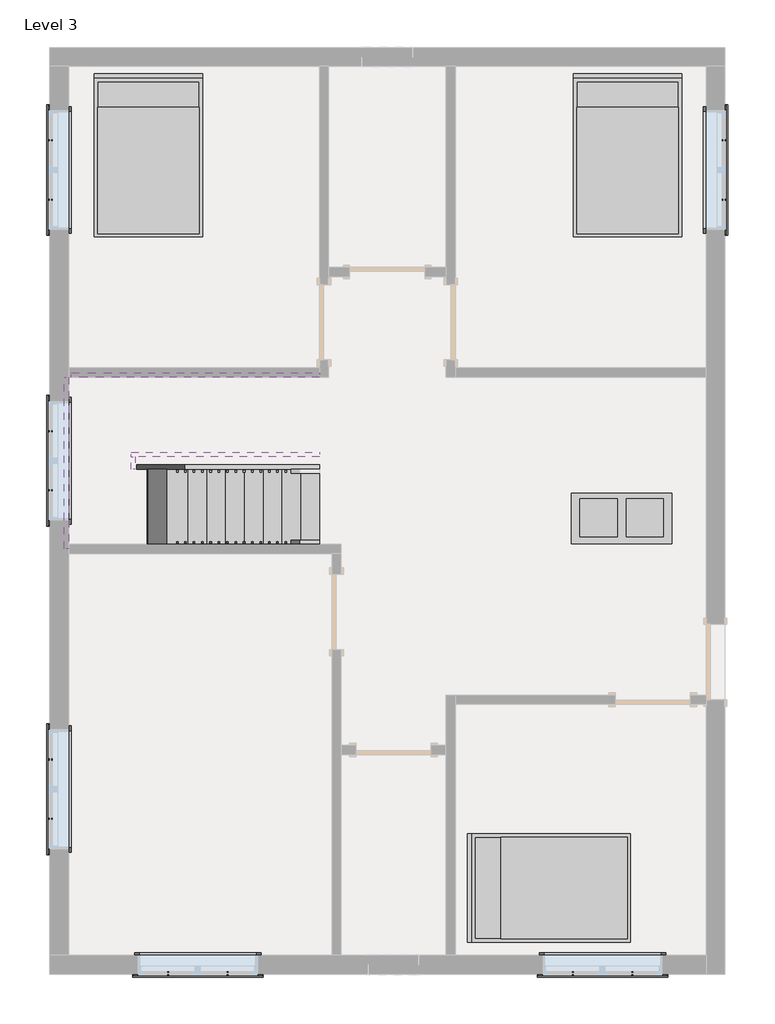
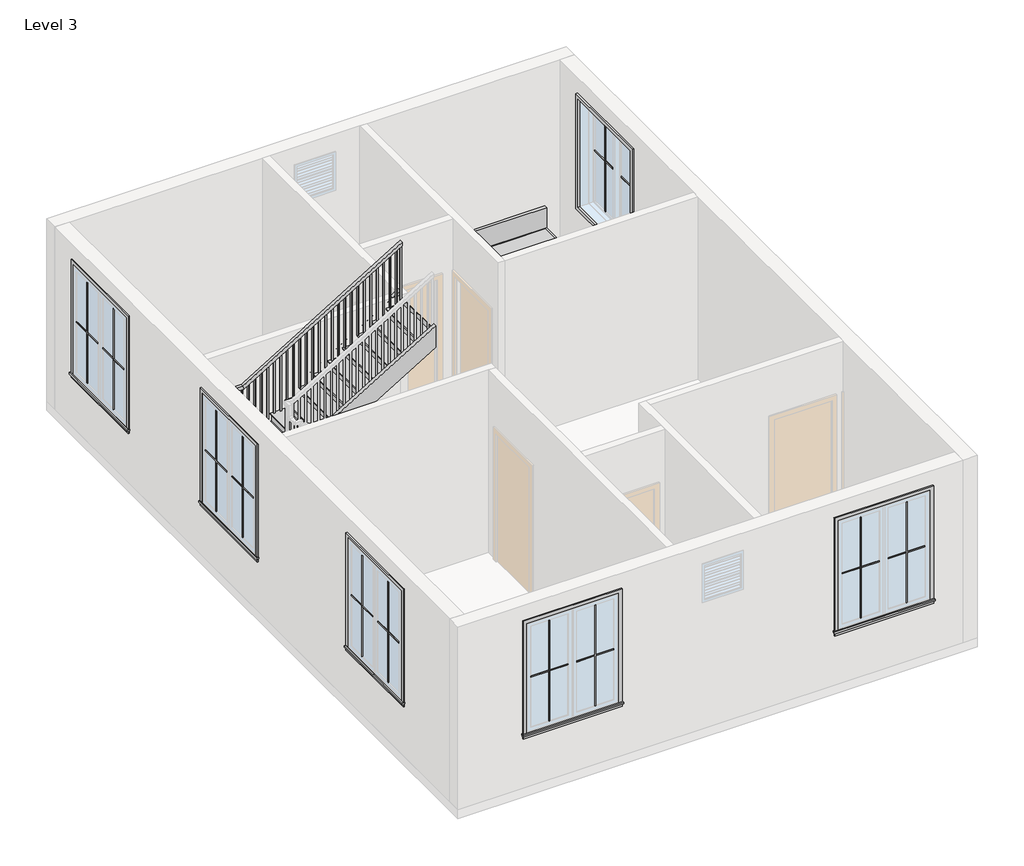
# One storey, part 2 of 2: 25 proxies, 6 members, 3 furniture elements, 1 railing, 1 stair flight.
"""IFC4 building model written with IfcOpenShell, lengths in millimetres."""

from ifc_helpers import new_model, si_unit, frame, origin, place, context, project, spatial, polyline, outline, extrude, faceted_brep, transform, mapped, element, save
from components import muntin_pattern_2x2_muntin_pattern_2x2_bff912c5, muntin_pattern_2x2_muntin_pattern_2x2_c2194282, trim_window_exterior_flat_with_sill_e04b3088, trim_window_interior_flat_picture_frame_2a7685fe, coffee_table_with_brass_mullions_11320_coffee_table_with_5962bef7, bed_17739_bed_17739_15c61121, stair_flight_ce5c0ca6

model = new_model("IFC4")

# Units and contexts
model_context = context("Model", 3, world=origin())
ifc_project = project(units=[si_unit("LENGTHUNIT", "METRE", prefix="MILLI")], contexts=[model_context])

# Site, building, storey
site = spatial("IfcSite", under=ifc_project)
building = spatial("IfcBuilding", under=site)
storey = spatial("IfcBuildingStorey", under=building, Name="Level 3", Elevation=3200.4)

# Proxies
placement = place(None, origin())
muntin_pattern_2x2_muntin_pattern_2x2_shape = muntin_pattern_2x2_muntin_pattern_2x2_bff912c5(model_context)
element("IfcBuildingElementProxy", 1, Name="Muntin Pattern_2x2 : Muntin Pattern_2x2", ObjectType="Muntin Pattern_2x2 : Muntin Pattern_2x2", at=placement, inside=storey, context=model_context, shape_type="MappedRepresentation", body=[
    mapped(muntin_pattern_2x2_muntin_pattern_2x2_shape, transform((-3196.8535855, -5792.3946383, 4184.65), x_axis=(-1.0, 0.0, 0.0), y_axis=(0.0, -1.0, 0.0), z_axis=(0.0, 0.0, 1.0))),
])
element("IfcBuildingElementProxy", 2, Name="Muntin Pattern_2x2 : Muntin Pattern_2x2", ObjectType="Muntin Pattern_2x2 : Muntin Pattern_2x2", at=placement, inside=storey, context=model_context, shape_type="MappedRepresentation", body=[
    mapped(muntin_pattern_2x2_muntin_pattern_2x2_shape, transform((-5347.9160855, -3914.3821383, 4184.65), x_axis=(0.0, 1.0, 0.0), y_axis=(-1.0, 0.0, 0.0), z_axis=(0.0, 0.0, 1.0))),
])
element("IfcBuildingElementProxy", 3, Name="Muntin Pattern_2x2 : Muntin Pattern_2x2", ObjectType="Muntin Pattern_2x2 : Muntin Pattern_2x2", at=placement, inside=storey, context=model_context, shape_type="MappedRepresentation", body=[
    mapped(muntin_pattern_2x2_muntin_pattern_2x2_shape, transform((1721.2214145, -5792.3946383, 4184.65), x_axis=(-1.0, 0.0, 0.0), y_axis=(0.0, -1.0, 0.0), z_axis=(0.0, 0.0, 1.0))),
])
element("IfcBuildingElementProxy", 4, Name="Muntin Pattern_2x2 : Muntin Pattern_2x2", ObjectType="Muntin Pattern_2x2 : Muntin Pattern_2x2", at=placement, inside=storey, context=model_context, shape_type="MappedRepresentation", body=[
    mapped(muntin_pattern_2x2_muntin_pattern_2x2_shape, transform((2837.2339145, 4324.7428617, 4184.65), x_axis=(0.0, -1.0, 0.0), y_axis=(1.0, 0.0, 0.0), z_axis=(0.0, 0.0, 1.0))),
])
element("IfcBuildingElementProxy", 5, Name="Muntin Pattern_2x2 : Muntin Pattern_2x2", ObjectType="Muntin Pattern_2x2 : Muntin Pattern_2x2", at=placement, inside=storey, context=model_context, shape_type="MappedRepresentation", body=[
    mapped(muntin_pattern_2x2_muntin_pattern_2x2_shape, transform((-5347.9160855, 3604.0178617, 4184.65), x_axis=(0.0, 1.0, 0.0), y_axis=(-1.0, 0.0, 0.0), z_axis=(0.0, 0.0, 1.0))),
])
element("IfcBuildingElementProxy", 6, Name="Muntin Pattern_2x2 : Muntin Pattern_2x2", ObjectType="Muntin Pattern_2x2 : Muntin Pattern_2x2", at=placement, inside=storey, context=model_context, shape_type="MappedRepresentation", body=[
    mapped(muntin_pattern_2x2_muntin_pattern_2x2_shape, transform((-5347.9160855, 73.4178617, 4184.65), x_axis=(0.0, 1.0, 0.0), y_axis=(-1.0, 0.0, 0.0), z_axis=(0.0, 0.0, 1.0))),
])
muntin_pattern_2x2_muntin_pattern_2x2_2_shape = muntin_pattern_2x2_muntin_pattern_2x2_c2194282(model_context)
element("IfcBuildingElementProxy", 7, Name="Muntin Pattern_2x2 : Muntin Pattern_2x2", ObjectType="Muntin Pattern_2x2 : Muntin Pattern_2x2", at=placement, inside=storey, context=model_context, shape_type="MappedRepresentation", body=[
    mapped(muntin_pattern_2x2_muntin_pattern_2x2_2_shape, transform((-3917.5785855, -5792.3946383, 4184.65), x_axis=(1.0, 0.0, 0.0), y_axis=(0.0, 1.0, 0.0), z_axis=(0.0, 0.0, 1.0))),
])
element("IfcBuildingElementProxy", 8, Name="Muntin Pattern_2x2 : Muntin Pattern_2x2", ObjectType="Muntin Pattern_2x2 : Muntin Pattern_2x2", at=placement, inside=storey, context=model_context, shape_type="MappedRepresentation", body=[
    mapped(muntin_pattern_2x2_muntin_pattern_2x2_2_shape, transform((-5347.9160855, -3193.6571383, 4184.65), x_axis=(0.0, -1.0, 0.0), y_axis=(1.0, 0.0, 0.0), z_axis=(0.0, 0.0, 1.0))),
])
element("IfcBuildingElementProxy", 9, Name="Muntin Pattern_2x2 : Muntin Pattern_2x2", ObjectType="Muntin Pattern_2x2 : Muntin Pattern_2x2", at=placement, inside=storey, context=model_context, shape_type="MappedRepresentation", body=[
    mapped(muntin_pattern_2x2_muntin_pattern_2x2_2_shape, transform((1000.4964145, -5792.3946383, 4184.65), x_axis=(1.0, 0.0, 0.0), y_axis=(0.0, 1.0, 0.0), z_axis=(0.0, 0.0, 1.0))),
])
element("IfcBuildingElementProxy", 10, Name="Muntin Pattern_2x2 : Muntin Pattern_2x2", ObjectType="Muntin Pattern_2x2 : Muntin Pattern_2x2", at=placement, inside=storey, context=model_context, shape_type="MappedRepresentation", body=[
    mapped(muntin_pattern_2x2_muntin_pattern_2x2_2_shape, transform((2837.2339145, 3604.0178617, 4184.65), x_axis=(0.0, 1.0, 0.0), y_axis=(-1.0, 0.0, 0.0), z_axis=(0.0, 0.0, 1.0))),
])
element("IfcBuildingElementProxy", 11, Name="Muntin Pattern_2x2 : Muntin Pattern_2x2", ObjectType="Muntin Pattern_2x2 : Muntin Pattern_2x2", at=placement, inside=storey, context=model_context, shape_type="MappedRepresentation", body=[
    mapped(muntin_pattern_2x2_muntin_pattern_2x2_2_shape, transform((-5347.9160855, 4324.7428617, 4184.65), x_axis=(0.0, -1.0, 0.0), y_axis=(1.0, 0.0, 0.0), z_axis=(0.0, 0.0, 1.0))),
])
element("IfcBuildingElementProxy", 12, Name="Muntin Pattern_2x2 : Muntin Pattern_2x2", ObjectType="Muntin Pattern_2x2 : Muntin Pattern_2x2", at=placement, inside=storey, context=model_context, shape_type="MappedRepresentation", body=[
    mapped(muntin_pattern_2x2_muntin_pattern_2x2_2_shape, transform((-5347.9160855, 794.1428617, 4184.65), x_axis=(0.0, -1.0, 0.0), y_axis=(1.0, 0.0, 0.0), z_axis=(0.0, 0.0, 1.0))),
])
trim_window_exterior_flat_with_sill_shape = trim_window_exterior_flat_with_sill_e04b3088(model_context)
element("IfcBuildingElementProxy", 13, Name="Trim-Window-Exterior-Flat : with Sill", ObjectType="Trim-Window-Exterior-Flat : with Sill", at=placement, inside=storey, context=model_context, shape_type="MappedRepresentation", body=[
    mapped(trim_window_exterior_flat_with_sill_shape, transform((-3557.2160855, -5801.9196383, 5943.6), x_axis=(1.0, 0.0, 0.0), y_axis=(0.0, 0.0, 1.0), z_axis=(0.0, -1.0, 0.0))),
])
element("IfcBuildingElementProxy", 14, Name="Trim-Window-Exterior-Flat : with Sill", ObjectType="Trim-Window-Exterior-Flat : with Sill", at=placement, inside=storey, context=model_context, shape_type="MappedRepresentation", body=[
    mapped(trim_window_exterior_flat_with_sill_shape, transform((-5357.4410855, -3554.0196383, 5943.6), x_axis=(0.0, -1.0, 0.0), y_axis=(0.0, 0.0, 1.0), z_axis=(-1.0, 0.0, 0.0))),
])
element("IfcBuildingElementProxy", 15, Name="Trim-Window-Exterior-Flat : with Sill", ObjectType="Trim-Window-Exterior-Flat : with Sill", at=placement, inside=storey, context=model_context, shape_type="MappedRepresentation", body=[
    mapped(trim_window_exterior_flat_with_sill_shape, transform((1360.8589145, -5801.9196383, 5943.6), x_axis=(1.0, 0.0, 0.0), y_axis=(0.0, 0.0, 1.0), z_axis=(0.0, -1.0, 0.0))),
])
element("IfcBuildingElementProxy", 16, Name="Trim-Window-Exterior-Flat : with Sill", ObjectType="Trim-Window-Exterior-Flat : with Sill", at=placement, inside=storey, context=model_context, shape_type="MappedRepresentation", body=[
    mapped(trim_window_exterior_flat_with_sill_shape, transform((2846.7589145, 3964.3803617, 5943.6), x_axis=(0.0, 1.0, 0.0), y_axis=(0.0, 0.0, 1.0), z_axis=(1.0, 0.0, 0.0))),
])
element("IfcBuildingElementProxy", 17, Name="Trim-Window-Exterior-Flat : with Sill", ObjectType="Trim-Window-Exterior-Flat : with Sill", at=placement, inside=storey, context=model_context, shape_type="MappedRepresentation", body=[
    mapped(trim_window_exterior_flat_with_sill_shape, transform((-5357.4410855, 3964.3803617, 5943.6), x_axis=(0.0, -1.0, 0.0), y_axis=(0.0, 0.0, 1.0), z_axis=(-1.0, 0.0, 0.0))),
])
element("IfcBuildingElementProxy", 18, Name="Trim-Window-Exterior-Flat : with Sill", ObjectType="Trim-Window-Exterior-Flat : with Sill", at=placement, inside=storey, context=model_context, shape_type="MappedRepresentation", body=[
    mapped(trim_window_exterior_flat_with_sill_shape, transform((-5357.4410855, 433.7803617, 5943.6), x_axis=(0.0, -1.0, 0.0), y_axis=(0.0, 0.0, 1.0), z_axis=(-1.0, 0.0, 0.0))),
])
trim_window_interior_flat_picture_frame_shape = trim_window_interior_flat_picture_frame_2a7685fe(model_context)
element("IfcBuildingElementProxy", 19, Name="Trim-Window-Interior-Flat : Picture Frame", ObjectType="Trim-Window-Interior-Flat : Picture Frame", at=placement, inside=storey, context=model_context, shape_type="MappedRepresentation", body=[
    mapped(trim_window_interior_flat_picture_frame_shape, transform((-3557.2160855, -5573.3196383, 5943.6), x_axis=(-1.0, 0.0, 0.0), y_axis=(0.0, 0.0, 1.0), z_axis=(0.0, 1.0, 0.0))),
])
element("IfcBuildingElementProxy", 20, Name="Trim-Window-Interior-Flat : Picture Frame", ObjectType="Trim-Window-Interior-Flat : Picture Frame", at=placement, inside=storey, context=model_context, shape_type="MappedRepresentation", body=[
    mapped(trim_window_interior_flat_picture_frame_shape, transform((-5128.8410855, -3554.0196383, 5943.6), x_axis=(0.0, 1.0, 0.0), y_axis=(0.0, 0.0, 1.0), z_axis=(1.0, 0.0, 0.0))),
])
element("IfcBuildingElementProxy", 21, Name="Trim-Window-Interior-Flat : Picture Frame", ObjectType="Trim-Window-Interior-Flat : Picture Frame", at=placement, inside=storey, context=model_context, shape_type="MappedRepresentation", body=[
    mapped(trim_window_interior_flat_picture_frame_shape, transform((1360.8589145, -5573.3196383, 5943.6), x_axis=(-1.0, 0.0, 0.0), y_axis=(0.0, 0.0, 1.0), z_axis=(0.0, 1.0, 0.0))),
])
element("IfcBuildingElementProxy", 22, Name="Trim-Window-Interior-Flat : Picture Frame", ObjectType="Trim-Window-Interior-Flat : Picture Frame", at=placement, inside=storey, context=model_context, shape_type="MappedRepresentation", body=[
    mapped(trim_window_interior_flat_picture_frame_shape, transform((2618.1589145, 3964.3803617, 5943.6), x_axis=(0.0, -1.0, 0.0), y_axis=(0.0, 0.0, 1.0), z_axis=(-1.0, 0.0, 0.0))),
])
element("IfcBuildingElementProxy", 23, Name="Trim-Window-Interior-Flat : Picture Frame", ObjectType="Trim-Window-Interior-Flat : Picture Frame", at=placement, inside=storey, context=model_context, shape_type="MappedRepresentation", body=[
    mapped(trim_window_interior_flat_picture_frame_shape, transform((-5128.8410855, 3964.3803617, 5943.6), x_axis=(0.0, 1.0, 0.0), y_axis=(0.0, 0.0, 1.0), z_axis=(1.0, 0.0, 0.0))),
])
element("IfcBuildingElementProxy", 24, Name="Trim-Window-Interior-Flat : Picture Frame", ObjectType="Trim-Window-Interior-Flat : Picture Frame", at=placement, inside=storey, context=model_context, shape_type="MappedRepresentation", body=[
    mapped(trim_window_interior_flat_picture_frame_shape, transform((-5128.8410855, 433.7803617, 5943.6), x_axis=(0.0, 1.0, 0.0), y_axis=(0.0, 0.0, 1.0), z_axis=(1.0, 0.0, 0.0))),
])
coffee_table_with_brass_mullions_11320_coffee_table_with_shape = coffee_table_with_brass_mullions_11320_coffee_table_with_5962bef7(model_context)
element("IfcBuildingElementProxy", 25, Name="coffee_table_with_brass_mullions_11320 : coffee_table_with_brass_mullions_11320", ObjectType="coffee_table_with_brass_mullions_11320 : coffee_table_with_brass_mullions_11320", at=placement, inside=storey, context=model_context, shape_type="MappedRepresentation", body=[
    mapped(coffee_table_with_brass_mullions_11320_coffee_table_with_shape, transform((2229.2258874, -696.5196383, 3200.4), x_axis=(1.0, 0.0, 0.0), y_axis=(0.0, 1.0, 0.0), z_axis=(0.0, 0.0, 1.0))),
])

# Furniture
bed_17739_bed_17739_shape = bed_17739_bed_17739_15c61121(model_context)
element("IfcFurniture", 26, ObjectType="Bed_17739 : Bed_17739", at=placement, inside=storey, context=model_context, shape_type="MappedRepresentation", body=[
    mapped(bed_17739_bed_17739_shape, transform((1665.6589145, 4116.7803617, 3200.4), x_axis=(1.0, 0.0, 0.0), y_axis=(0.0, 1.0, 0.0), z_axis=(0.0, 0.0, 1.0))),
])
element("IfcFurniture", 27, ObjectType="Bed_17739 : Bed_17739", at=placement, inside=storey, context=model_context, shape_type="MappedRepresentation", body=[
    mapped(bed_17739_bed_17739_shape, transform((-4157.2910855, 4116.7803617, 3200.4), x_axis=(1.0, 0.0, 0.0), y_axis=(0.0, 1.0, 0.0), z_axis=(0.0, 0.0, 1.0))),
])
element("IfcFurniture", 28, ObjectType="Bed_17739 : Bed_17739", at=placement, inside=storey, context=model_context, shape_type="MappedRepresentation", body=[
    mapped(bed_17739_bed_17739_shape, transform((732.2089145, -4754.5725945, 3200.4), x_axis=(0.0, 1.0, 0.0), y_axis=(-1.0, 0.0, 0.0), z_axis=(0.0, 0.0, 1.0))),
])

# Members
element("IfcMember", 29, ObjectType="Stringer - 2\" Width", at=placement, inside=storey, context=model_context, shape_type="SweptSolid", body=[
    extrude(outline(polyline([(3200.4, -2080.8410855), (3412.514512, -2080.8410855), (4800.6, -4371.1821407), (4800.6, -4959.2565972), (3200.4, -2318.9265972), (3200.4, -2080.8410855)])), frame((0.0, -633.0196383, 0.0), z_axis=(0.0, 1.0, 0.0), x_axis=(0.0, 0.0, 1.0)), (0.0, 0.0, 1.0), 50.8),
])
element("IfcMember", 30, ObjectType="Stringer - 2\" Width", at=placement, inside=storey, context=model_context, shape_type="SweptSolid", body=[
    extrude(outline(polyline([(-5128.8410855, -633.0196383), (-5179.6410855, -633.0196383), (-5179.6410855, 1449.7803617), (-5128.8410855, 1449.7803617), (-5128.8410855, -633.0196383)])), frame((0.0, 0.0, 4495.8), z_axis=(0.0, 0.0, 1.0), x_axis=(1.0, 0.0, 0.0)), (0.0, 0.0, 1.0), 304.8),
])
element("IfcMember", 31, ObjectType="Stringer - 2\" Width", at=placement, inside=storey, context=model_context, shape_type="SweptSolid", body=[
    extrude(outline(polyline([(4495.8, -4505.9455737), (5965.5602959, -2080.8410855), (6321.9690574, -2080.8410855), (4495.8, -5094.0200302), (4495.8, -4505.9455737)])), frame((0.0, 1449.7803617, 0.0), z_axis=(0.0, 1.0, 0.0), x_axis=(0.0, 0.0, 1.0)), (0.0, 0.0, 1.0), 50.8),
])
element("IfcMember", 32, ObjectType="Stringer - 2\" Width", at=placement, inside=storey, context=model_context, shape_type="SweptSolid", body=[
    extrude(outline(polyline([(3200.4, -2080.8410855), (3412.514512, -2080.8410855), (4767.1811786, -4316.0410855), (4410.7724171, -4316.0410855), (3200.4, -2318.9265972), (3200.4, -2080.8410855)])), frame((0.0, 332.1803617, 0.0), z_axis=(0.0, 1.0, 0.0), x_axis=(0.0, 0.0, 1.0)), (0.0, 0.0, 1.0), 50.8),
])
element("IfcMember", 33, ObjectType="Stringer - 2\" Width", at=placement, inside=storey, context=model_context, shape_type="SweptSolid", body=[
    extrude(outline(polyline([(-4316.0410855, 332.1803617), (-4366.8410855, 332.1803617), (-4366.8410855, 484.5803617), (-4316.0410855, 484.5803617), (-4316.0410855, 332.1803617)])), frame((0.0, 0.0, 4495.8), z_axis=(0.0, 0.0, 1.0), x_axis=(1.0, 0.0, 0.0)), (0.0, 0.0, 1.0), 304.8),
])
element("IfcMember", 34, ObjectType="Stringer - 2\" Width", at=placement, inside=storey, context=model_context, shape_type="SweptSolid", body=[
    extrude(outline(polyline([(4936.514512, -4366.8410855), (4580.1057504, -4366.8410855), (5965.5602959, -2080.8410855), (6321.9690574, -2080.8410855), (4936.514512, -4366.8410855)])), frame((0.0, 484.5803617, 0.0), z_axis=(0.0, 1.0, 0.0), x_axis=(0.0, 0.0, 1.0)), (0.0, 0.0, 1.0), 50.8),
])

# Railing
element("IfcRailing", 35, ObjectType="Handrail - Rectangular", at=placement, inside=storey, context=model_context, shape_type="SolidModel", body=[
    faceted_brep([(-2080.8410855, -582.2196383, 4253.3454545), (-2080.8410855, -582.2196383, 4193.9439943), (-2080.8410855, -531.4196383, 4193.9439943), (-2080.8410855, -531.4196383, 4253.3454545), (-4366.8410855, -582.2196383, 5638.8), (-4381.0334949, -582.2196383, 5588.0), (-4381.0334949, -531.4196383, 5588.0), (-4366.8410855, -531.4196383, 5638.8), (-5128.8410855, -582.2196383, 5638.8), (-5128.8410855, -582.2196383, 5588.0), (-5078.0410855, -531.4196383, 5588.0), (-5078.0410855, -531.4196383, 5638.8), (-5128.8410855, 1449.7803617, 5638.8), (-5128.8410855, 1449.7803617, 5588.0), (-5078.0410855, 1398.9803617, 5588.0), (-5078.0410855, 1398.9803617, 5638.8), (-4595.4410855, 1449.7803617, 5638.8), (-4581.2486761, 1449.7803617, 5588.0), (-4581.2486761, 1398.9803617, 5588.0), (-4595.4410855, 1398.9803617, 5638.8), (-2080.8410855, 1449.7803617, 7162.8), (-2080.8410855, 1398.9803617, 7162.8), (-2080.8410855, 1398.9803617, 7103.3985397), (-2080.8410855, 1449.7803617, 7103.3985397)], [[[0, 1, 2, 3]], [[1, 0, 4, 5]], [[2, 1, 5, 6]], [[3, 2, 6, 7]], [[0, 3, 7, 4]], [[5, 4, 8, 9]], [[6, 5, 9, 10]], [[7, 6, 10, 11]], [[4, 7, 11, 8]], [[9, 8, 12, 13]], [[10, 9, 13, 14]], [[11, 10, 14, 15]], [[8, 11, 15, 12]], [[13, 12, 16, 17]], [[14, 13, 17, 18]], [[15, 14, 18, 19]], [[12, 15, 19, 16]], [[20, 21, 22, 23]], [[17, 16, 20, 23]], [[18, 17, 23, 22]], [[19, 18, 22, 21]], [[16, 19, 21, 20]]]),
    extrude(outline(polyline([(7051.4439943, -2166.5660855), (6109.8545455, -2166.5660855), (6109.8545455, -2147.5160855), (7062.9894488, -2147.5160855), (7051.4439943, -2166.5660855)])), frame((0.0, 1414.8553617, 0.0), z_axis=(0.0, 1.0, 0.0), x_axis=(0.0, 0.0, 1.0)), (0.0, 0.0, 1.0), 19.05),
    extrude(outline(polyline([(6989.8682367, -2268.1660855), (6109.8545455, -2268.1660855), (6109.8545455, -2249.1160855), (7001.4136913, -2249.1160855), (6989.8682367, -2268.1660855)])), frame((0.0, 1414.8553617, 0.0), z_axis=(0.0, 1.0, 0.0), x_axis=(0.0, 0.0, 1.0)), (0.0, 0.0, 1.0), 19.05),
    extrude(outline(polyline([(6928.2924791, -2369.7660855), (5971.3090909, -2369.7660855), (5971.3090909, -2350.7160855), (6939.8379337, -2350.7160855), (6928.2924791, -2369.7660855)])), frame((0.0, 1414.8553617, 0.0), z_axis=(0.0, 1.0, 0.0), x_axis=(0.0, 0.0, 1.0)), (0.0, 0.0, 1.0), 19.05),
    extrude(outline(polyline([(6866.7167216, -2471.3660855), (5971.3090909, -2471.3660855), (5971.3090909, -2452.3160855), (6878.2621761, -2452.3160855), (6866.7167216, -2471.3660855)])), frame((0.0, 1414.8553617, 0.0), z_axis=(0.0, 1.0, 0.0), x_axis=(0.0, 0.0, 1.0)), (0.0, 0.0, 1.0), 19.05),
    extrude(outline(polyline([(6805.140964, -2572.9660855), (5832.7636364, -2572.9660855), (5832.7636364, -2553.9160855), (6816.6864185, -2553.9160855), (6805.140964, -2572.9660855)])), frame((0.0, 1414.8553617, 0.0), z_axis=(0.0, 1.0, 0.0), x_axis=(0.0, 0.0, 1.0)), (0.0, 0.0, 1.0), 19.05),
    extrude(outline(polyline([(6743.5652064, -2674.5660855), (5832.7636364, -2674.5660855), (5832.7636364, -2655.5160855), (6755.110661, -2655.5160855), (6743.5652064, -2674.5660855)])), frame((0.0, 1414.8553617, 0.0), z_axis=(0.0, 1.0, 0.0), x_axis=(0.0, 0.0, 1.0)), (0.0, 0.0, 1.0), 19.05),
    extrude(outline(polyline([(6681.9894488, -2776.1660855), (5832.7636364, -2776.1660855), (5832.7636364, -2757.1160855), (6693.5349034, -2757.1160855), (6681.9894488, -2776.1660855)])), frame((0.0, 1414.8553617, 0.0), z_axis=(0.0, 1.0, 0.0), x_axis=(0.0, 0.0, 1.0)), (0.0, 0.0, 1.0), 19.05),
    extrude(outline(polyline([(6620.4136913, -2877.7660855), (5694.2181818, -2877.7660855), (5694.2181818, -2858.7160855), (6631.9591458, -2858.7160855), (6620.4136913, -2877.7660855)])), frame((0.0, 1414.8553617, 0.0), z_axis=(0.0, 1.0, 0.0), x_axis=(0.0, 0.0, 1.0)), (0.0, 0.0, 1.0), 19.05),
    extrude(outline(polyline([(6558.8379337, -2979.3660855), (5694.2181818, -2979.3660855), (5694.2181818, -2960.3160855), (6570.3833882, -2960.3160855), (6558.8379337, -2979.3660855)])), frame((0.0, 1414.8553617, 0.0), z_axis=(0.0, 1.0, 0.0), x_axis=(0.0, 0.0, 1.0)), (0.0, 0.0, 1.0), 19.05),
    extrude(outline(polyline([(6497.2621761, -3080.9660855), (5555.6727273, -3080.9660855), (5555.6727273, -3061.9160855), (6508.8076307, -3061.9160855), (6497.2621761, -3080.9660855)])), frame((0.0, 1414.8553617, 0.0), z_axis=(0.0, 1.0, 0.0), x_axis=(0.0, 0.0, 1.0)), (0.0, 0.0, 1.0), 19.05),
    extrude(outline(polyline([(6435.6864185, -3182.5660855), (5555.6727273, -3182.5660855), (5555.6727273, -3163.5160855), (6447.2318731, -3163.5160855), (6435.6864185, -3182.5660855)])), frame((0.0, 1414.8553617, 0.0), z_axis=(0.0, 1.0, 0.0), x_axis=(0.0, 0.0, 1.0)), (0.0, 0.0, 1.0), 19.05),
    extrude(outline(polyline([(6374.110661, -3284.1660855), (5417.1272727, -3284.1660855), (5417.1272727, -3265.1160855), (6385.6561155, -3265.1160855), (6374.110661, -3284.1660855)])), frame((0.0, 1414.8553617, 0.0), z_axis=(0.0, 1.0, 0.0), x_axis=(0.0, 0.0, 1.0)), (0.0, 0.0, 1.0), 19.05),
    extrude(outline(polyline([(6312.5349034, -3385.7660855), (5417.1272727, -3385.7660855), (5417.1272727, -3366.7160855), (6324.0803579, -3366.7160855), (6312.5349034, -3385.7660855)])), frame((0.0, 1414.8553617, 0.0), z_axis=(0.0, 1.0, 0.0), x_axis=(0.0, 0.0, 1.0)), (0.0, 0.0, 1.0), 19.05),
    extrude(outline(polyline([(6250.9591458, -3487.3660855), (5278.5818182, -3487.3660855), (5278.5818182, -3468.3160855), (6262.5046004, -3468.3160855), (6250.9591458, -3487.3660855)])), frame((0.0, 1414.8553617, 0.0), z_axis=(0.0, 1.0, 0.0), x_axis=(0.0, 0.0, 1.0)), (0.0, 0.0, 1.0), 19.05),
    extrude(outline(polyline([(6189.3833882, -3588.9660855), (5278.5818182, -3588.9660855), (5278.5818182, -3569.9160855), (6200.9288428, -3569.9160855), (6189.3833882, -3588.9660855)])), frame((0.0, 1414.8553617, 0.0), z_axis=(0.0, 1.0, 0.0), x_axis=(0.0, 0.0, 1.0)), (0.0, 0.0, 1.0), 19.05),
    extrude(outline(polyline([(6127.8076307, -3690.5660855), (5278.5818182, -3690.5660855), (5278.5818182, -3671.5160855), (6139.3530852, -3671.5160855), (6127.8076307, -3690.5660855)])), frame((0.0, 1414.8553617, 0.0), z_axis=(0.0, 1.0, 0.0), x_axis=(0.0, 0.0, 1.0)), (0.0, 0.0, 1.0), 19.05),
    extrude(outline(polyline([(6066.2318731, -3792.1660855), (5140.0363636, -3792.1660855), (5140.0363636, -3773.1160855), (6077.7773276, -3773.1160855), (6066.2318731, -3792.1660855)])), frame((0.0, 1414.8553617, 0.0), z_axis=(0.0, 1.0, 0.0), x_axis=(0.0, 0.0, 1.0)), (0.0, 0.0, 1.0), 19.05),
    extrude(outline(polyline([(6004.6561155, -3893.7660855), (5140.0363636, -3893.7660855), (5140.0363636, -3874.7160855), (6016.20157, -3874.7160855), (6004.6561155, -3893.7660855)])), frame((0.0, 1414.8553617, 0.0), z_axis=(0.0, 1.0, 0.0), x_axis=(0.0, 0.0, 1.0)), (0.0, 0.0, 1.0), 19.05),
    extrude(outline(polyline([(5943.0803579, -3995.3660855), (5001.4909091, -3995.3660855), (5001.4909091, -3976.3160855), (5954.6258125, -3976.3160855), (5943.0803579, -3995.3660855)])), frame((0.0, 1414.8553617, 0.0), z_axis=(0.0, 1.0, 0.0), x_axis=(0.0, 0.0, 1.0)), (0.0, 0.0, 1.0), 19.05),
    extrude(outline(polyline([(5881.5046004, -4096.9660855), (5001.4909091, -4096.9660855), (5001.4909091, -4077.9160855), (5893.0500549, -4077.9160855), (5881.5046004, -4096.9660855)])), frame((0.0, 1414.8553617, 0.0), z_axis=(0.0, 1.0, 0.0), x_axis=(0.0, 0.0, 1.0)), (0.0, 0.0, 1.0), 19.05),
    extrude(outline(polyline([(5819.9288428, -4198.5660855), (4862.9454545, -4198.5660855), (4862.9454545, -4179.5160855), (5831.4742973, -4179.5160855), (5819.9288428, -4198.5660855)])), frame((0.0, 1414.8553617, 0.0), z_axis=(0.0, 1.0, 0.0), x_axis=(0.0, 0.0, 1.0)), (0.0, 0.0, 1.0), 19.05),
    extrude(outline(polyline([(5758.3530852, -4300.1660855), (4862.9454545, -4300.1660855), (4862.9454545, -4281.1160855), (5769.8985397, -4281.1160855), (5758.3530852, -4300.1660855)])), frame((0.0, 1414.8553617, 0.0), z_axis=(0.0, 1.0, 0.0), x_axis=(0.0, 0.0, 1.0)), (0.0, 0.0, 1.0), 19.05),
    extrude(outline(polyline([(5696.7773276, -4401.7660855), (4724.4, -4401.7660855), (4724.4, -4382.7160855), (5708.3227822, -4382.7160855), (5696.7773276, -4401.7660855)])), frame((0.0, 1414.8553617, 0.0), z_axis=(0.0, 1.0, 0.0), x_axis=(0.0, 0.0, 1.0)), (0.0, 0.0, 1.0), 19.05),
    extrude(outline(polyline([(5635.20157, -4503.3660855), (4724.4, -4503.3660855), (4724.4, -4484.3160855), (5646.7470246, -4484.3160855), (5635.20157, -4503.3660855)])), frame((0.0, 1414.8553617, 0.0), z_axis=(0.0, 1.0, 0.0), x_axis=(0.0, 0.0, 1.0)), (0.0, 0.0, 1.0), 19.05),
    extrude(outline(polyline([(-4604.9660855, 1433.9053617), (-4585.9160855, 1433.9053617), (-4585.9160855, 1414.8553617), (-4604.9660855, 1414.8553617), (-4604.9660855, 1433.9053617)])), frame((0.0, 0.0, 4724.4), z_axis=(0.0, 0.0, 1.0), x_axis=(1.0, 0.0, 0.0)), (0.0, 0.0, 1.0), 863.6),
    extrude(outline(polyline([(-4706.5660855, 1433.9053617), (-4687.5160855, 1433.9053617), (-4687.5160855, 1414.8553617), (-4706.5660855, 1414.8553617), (-4706.5660855, 1433.9053617)])), frame((0.0, 0.0, 4724.4), z_axis=(0.0, 0.0, 1.0), x_axis=(1.0, 0.0, 0.0)), (0.0, 0.0, 1.0), 863.6),
    extrude(outline(polyline([(-4808.1660855, 1433.9053617), (-4789.1160855, 1433.9053617), (-4789.1160855, 1414.8553617), (-4808.1660855, 1414.8553617), (-4808.1660855, 1433.9053617)])), frame((0.0, 0.0, 4724.4), z_axis=(0.0, 0.0, 1.0), x_axis=(1.0, 0.0, 0.0)), (0.0, 0.0, 1.0), 863.6),
    extrude(outline(polyline([(-4909.7660855, 1433.9053617), (-4890.7160855, 1433.9053617), (-4890.7160855, 1414.8553617), (-4909.7660855, 1414.8553617), (-4909.7660855, 1433.9053617)])), frame((0.0, 0.0, 4724.4), z_axis=(0.0, 0.0, 1.0), x_axis=(1.0, 0.0, 0.0)), (0.0, 0.0, 1.0), 863.6),
    extrude(outline(polyline([(-5011.3660855, 1433.9053617), (-4992.3160855, 1433.9053617), (-4992.3160855, 1414.8553617), (-5011.3660855, 1414.8553617), (-5011.3660855, 1433.9053617)])), frame((0.0, 0.0, 4724.4), z_axis=(0.0, 0.0, 1.0), x_axis=(1.0, 0.0, 0.0)), (0.0, 0.0, 1.0), 863.6),
    extrude(outline(polyline([(-5112.9660855, 1364.0553617), (-5112.9660855, 1383.1053617), (-5093.9160855, 1383.1053617), (-5093.9160855, 1364.0553617), (-5112.9660855, 1364.0553617)])), frame((0.0, 0.0, 4724.4), z_axis=(0.0, 0.0, 1.0), x_axis=(1.0, 0.0, 0.0)), (0.0, 0.0, 1.0), 863.6),
    extrude(outline(polyline([(-5112.9660855, 1262.4553617), (-5112.9660855, 1281.5053617), (-5093.9160855, 1281.5053617), (-5093.9160855, 1262.4553617), (-5112.9660855, 1262.4553617)])), frame((0.0, 0.0, 4724.4), z_axis=(0.0, 0.0, 1.0), x_axis=(1.0, 0.0, 0.0)), (0.0, 0.0, 1.0), 863.6),
    extrude(outline(polyline([(-5112.9660855, 1160.8553617), (-5112.9660855, 1179.9053617), (-5093.9160855, 1179.9053617), (-5093.9160855, 1160.8553617), (-5112.9660855, 1160.8553617)])), frame((0.0, 0.0, 4724.4), z_axis=(0.0, 0.0, 1.0), x_axis=(1.0, 0.0, 0.0)), (0.0, 0.0, 1.0), 863.6),
    extrude(outline(polyline([(-5112.9660855, 1059.2553617), (-5112.9660855, 1078.3053617), (-5093.9160855, 1078.3053617), (-5093.9160855, 1059.2553617), (-5112.9660855, 1059.2553617)])), frame((0.0, 0.0, 4724.4), z_axis=(0.0, 0.0, 1.0), x_axis=(1.0, 0.0, 0.0)), (0.0, 0.0, 1.0), 863.6),
    extrude(outline(polyline([(-5112.9660855, 957.6553617), (-5112.9660855, 976.7053617), (-5093.9160855, 976.7053617), (-5093.9160855, 957.6553617), (-5112.9660855, 957.6553617)])), frame((0.0, 0.0, 4724.4), z_axis=(0.0, 0.0, 1.0), x_axis=(1.0, 0.0, 0.0)), (0.0, 0.0, 1.0), 863.6),
    extrude(outline(polyline([(-5112.9660855, 856.0553617), (-5112.9660855, 875.1053617), (-5093.9160855, 875.1053617), (-5093.9160855, 856.0553617), (-5112.9660855, 856.0553617)])), frame((0.0, 0.0, 4724.4), z_axis=(0.0, 0.0, 1.0), x_axis=(1.0, 0.0, 0.0)), (0.0, 0.0, 1.0), 863.6),
    extrude(outline(polyline([(-5112.9660855, 754.4553617), (-5112.9660855, 773.5053617), (-5093.9160855, 773.5053617), (-5093.9160855, 754.4553617), (-5112.9660855, 754.4553617)])), frame((0.0, 0.0, 4724.4), z_axis=(0.0, 0.0, 1.0), x_axis=(1.0, 0.0, 0.0)), (0.0, 0.0, 1.0), 863.6),
    extrude(outline(polyline([(-5112.9660855, 652.8553617), (-5112.9660855, 671.9053617), (-5093.9160855, 671.9053617), (-5093.9160855, 652.8553617), (-5112.9660855, 652.8553617)])), frame((0.0, 0.0, 4724.4), z_axis=(0.0, 0.0, 1.0), x_axis=(1.0, 0.0, 0.0)), (0.0, 0.0, 1.0), 863.6),
    extrude(outline(polyline([(-5112.9660855, 551.2553617), (-5112.9660855, 570.3053617), (-5093.9160855, 570.3053617), (-5093.9160855, 551.2553617), (-5112.9660855, 551.2553617)])), frame((0.0, 0.0, 4724.4), z_axis=(0.0, 0.0, 1.0), x_axis=(1.0, 0.0, 0.0)), (0.0, 0.0, 1.0), 863.6),
    extrude(outline(polyline([(-5112.9660855, 449.6553617), (-5112.9660855, 468.7053617), (-5093.9160855, 468.7053617), (-5093.9160855, 449.6553617), (-5112.9660855, 449.6553617)])), frame((0.0, 0.0, 4724.4), z_axis=(0.0, 0.0, 1.0), x_axis=(1.0, 0.0, 0.0)), (0.0, 0.0, 1.0), 863.6),
    extrude(outline(polyline([(-5112.9660855, 348.0553617), (-5112.9660855, 367.1053617), (-5093.9160855, 367.1053617), (-5093.9160855, 348.0553617), (-5112.9660855, 348.0553617)])), frame((0.0, 0.0, 4724.4), z_axis=(0.0, 0.0, 1.0), x_axis=(1.0, 0.0, 0.0)), (0.0, 0.0, 1.0), 863.6),
    extrude(outline(polyline([(-5112.9660855, 246.4553617), (-5112.9660855, 265.5053617), (-5093.9160855, 265.5053617), (-5093.9160855, 246.4553617), (-5112.9660855, 246.4553617)])), frame((0.0, 0.0, 4724.4), z_axis=(0.0, 0.0, 1.0), x_axis=(1.0, 0.0, 0.0)), (0.0, 0.0, 1.0), 863.6),
    extrude(outline(polyline([(-5112.9660855, 144.8553617), (-5112.9660855, 163.9053617), (-5093.9160855, 163.9053617), (-5093.9160855, 144.8553617), (-5112.9660855, 144.8553617)])), frame((0.0, 0.0, 4724.4), z_axis=(0.0, 0.0, 1.0), x_axis=(1.0, 0.0, 0.0)), (0.0, 0.0, 1.0), 863.6),
    extrude(outline(polyline([(-5112.9660855, 43.2553617), (-5112.9660855, 62.3053617), (-5093.9160855, 62.3053617), (-5093.9160855, 43.2553617), (-5112.9660855, 43.2553617)])), frame((0.0, 0.0, 4724.4), z_axis=(0.0, 0.0, 1.0), x_axis=(1.0, 0.0, 0.0)), (0.0, 0.0, 1.0), 863.6),
    extrude(outline(polyline([(-5112.9660855, -58.3446383), (-5112.9660855, -39.2946383), (-5093.9160855, -39.2946383), (-5093.9160855, -58.3446383), (-5112.9660855, -58.3446383)])), frame((0.0, 0.0, 4724.4), z_axis=(0.0, 0.0, 1.0), x_axis=(1.0, 0.0, 0.0)), (0.0, 0.0, 1.0), 863.6),
    extrude(outline(polyline([(-5112.9660855, -159.9446383), (-5112.9660855, -140.8946383), (-5093.9160855, -140.8946383), (-5093.9160855, -159.9446383), (-5112.9660855, -159.9446383)])), frame((0.0, 0.0, 4724.4), z_axis=(0.0, 0.0, 1.0), x_axis=(1.0, 0.0, 0.0)), (0.0, 0.0, 1.0), 863.6),
    extrude(outline(polyline([(-5112.9660855, -261.5446383), (-5112.9660855, -242.4946383), (-5093.9160855, -242.4946383), (-5093.9160855, -261.5446383), (-5112.9660855, -261.5446383)])), frame((0.0, 0.0, 4724.4), z_axis=(0.0, 0.0, 1.0), x_axis=(1.0, 0.0, 0.0)), (0.0, 0.0, 1.0), 863.6),
    extrude(outline(polyline([(-5112.9660855, -363.1446383), (-5112.9660855, -344.0946383), (-5093.9160855, -344.0946383), (-5093.9160855, -363.1446383), (-5112.9660855, -363.1446383)])), frame((0.0, 0.0, 4724.4), z_axis=(0.0, 0.0, 1.0), x_axis=(1.0, 0.0, 0.0)), (0.0, 0.0, 1.0), 863.6),
    extrude(outline(polyline([(-5112.9660855, -464.7446383), (-5112.9660855, -445.6946383), (-5093.9160855, -445.6946383), (-5093.9160855, -464.7446383), (-5112.9660855, -464.7446383)])), frame((0.0, 0.0, 4724.4), z_axis=(0.0, 0.0, 1.0), x_axis=(1.0, 0.0, 0.0)), (0.0, 0.0, 1.0), 863.6),
    extrude(outline(polyline([(-5017.7160855, -566.3446383), (-5036.7660855, -566.3446383), (-5036.7660855, -547.2946383), (-5017.7160855, -547.2946383), (-5017.7160855, -566.3446383)])), frame((0.0, 0.0, 4724.4), z_axis=(0.0, 0.0, 1.0), x_axis=(1.0, 0.0, 0.0)), (0.0, 0.0, 1.0), 863.6),
    extrude(outline(polyline([(-4916.1160855, -566.3446383), (-4935.1660855, -566.3446383), (-4935.1660855, -547.2946383), (-4916.1160855, -547.2946383), (-4916.1160855, -566.3446383)])), frame((0.0, 0.0, 4724.4), z_axis=(0.0, 0.0, 1.0), x_axis=(1.0, 0.0, 0.0)), (0.0, 0.0, 1.0), 863.6),
    extrude(outline(polyline([(-4814.5160855, -566.3446383), (-4833.5660855, -566.3446383), (-4833.5660855, -547.2946383), (-4814.5160855, -547.2946383), (-4814.5160855, -566.3446383)])), frame((0.0, 0.0, 4724.4), z_axis=(0.0, 0.0, 1.0), x_axis=(1.0, 0.0, 0.0)), (0.0, 0.0, 1.0), 863.6),
    extrude(outline(polyline([(-4712.9160855, -566.3446383), (-4731.9660855, -566.3446383), (-4731.9660855, -547.2946383), (-4712.9160855, -547.2946383), (-4712.9160855, -566.3446383)])), frame((0.0, 0.0, 4724.4), z_axis=(0.0, 0.0, 1.0), x_axis=(1.0, 0.0, 0.0)), (0.0, 0.0, 1.0), 863.6),
    extrude(outline(polyline([(-4611.3160855, -566.3446383), (-4630.3660855, -566.3446383), (-4630.3660855, -547.2946383), (-4611.3160855, -547.2946383), (-4611.3160855, -566.3446383)])), frame((0.0, 0.0, 4724.4), z_axis=(0.0, 0.0, 1.0), x_axis=(1.0, 0.0, 0.0)), (0.0, 0.0, 1.0), 863.6),
    extrude(outline(polyline([(-4509.7160855, -566.3446383), (-4528.7660855, -566.3446383), (-4528.7660855, -547.2946383), (-4509.7160855, -547.2946383), (-4509.7160855, -566.3446383)])), frame((0.0, 0.0, 4724.4), z_axis=(0.0, 0.0, 1.0), x_axis=(1.0, 0.0, 0.0)), (0.0, 0.0, 1.0), 863.6),
    extrude(outline(polyline([(-4408.1160855, -566.3446383), (-4427.1660855, -566.3446383), (-4427.1660855, -547.2946383), (-4408.1160855, -547.2946383), (-4408.1160855, -566.3446383)])), frame((0.0, 0.0, 4724.4), z_axis=(0.0, 0.0, 1.0), x_axis=(1.0, 0.0, 0.0)), (0.0, 0.0, 1.0), 863.6),
    extrude(outline(polyline([(5554.3833882, -4325.5660855), (4585.8545455, -4325.5660855), (4585.8545455, -4306.5160855), (5542.8379337, -4306.5160855), (5554.3833882, -4325.5660855)])), frame((0.0, -566.3446383, 0.0), z_axis=(0.0, 1.0, 0.0), x_axis=(0.0, 0.0, 1.0)), (0.0, 0.0, 1.0), 19.05),
    extrude(outline(polyline([(5492.8076307, -4223.9660855), (4585.8545455, -4223.9660855), (4585.8545455, -4204.9160855), (5481.2621761, -4204.9160855), (5492.8076307, -4223.9660855)])), frame((0.0, -566.3446383, 0.0), z_axis=(0.0, 1.0, 0.0), x_axis=(0.0, 0.0, 1.0)), (0.0, 0.0, 1.0), 19.05),
    extrude(outline(polyline([(5431.2318731, -4122.3660855), (4447.3090909, -4122.3660855), (4447.3090909, -4103.3160855), (5419.6864185, -4103.3160855), (5431.2318731, -4122.3660855)])), frame((0.0, -566.3446383, 0.0), z_axis=(0.0, 1.0, 0.0), x_axis=(0.0, 0.0, 1.0)), (0.0, 0.0, 1.0), 19.05),
    extrude(outline(polyline([(5369.6561155, -4020.7660855), (4447.3090909, -4020.7660855), (4447.3090909, -4001.7160855), (5358.110661, -4001.7160855), (5369.6561155, -4020.7660855)])), frame((0.0, -566.3446383, 0.0), z_axis=(0.0, 1.0, 0.0), x_axis=(0.0, 0.0, 1.0)), (0.0, 0.0, 1.0), 19.05),
    extrude(outline(polyline([(5308.0803579, -3919.1660855), (4447.3090909, -3919.1660855), (4447.3090909, -3900.1160855), (5296.5349034, -3900.1160855), (5308.0803579, -3919.1660855)])), frame((0.0, -566.3446383, 0.0), z_axis=(0.0, 1.0, 0.0), x_axis=(0.0, 0.0, 1.0)), (0.0, 0.0, 1.0), 19.05),
    extrude(outline(polyline([(5246.5046004, -3817.5660855), (4308.7636364, -3817.5660855), (4308.7636364, -3798.5160855), (5234.9591458, -3798.5160855), (5246.5046004, -3817.5660855)])), frame((0.0, -566.3446383, 0.0), z_axis=(0.0, 1.0, 0.0), x_axis=(0.0, 0.0, 1.0)), (0.0, 0.0, 1.0), 19.05),
    extrude(outline(polyline([(5184.9288428, -3715.9660855), (4308.7636364, -3715.9660855), (4308.7636364, -3696.9160855), (5173.3833882, -3696.9160855), (5184.9288428, -3715.9660855)])), frame((0.0, -566.3446383, 0.0), z_axis=(0.0, 1.0, 0.0), x_axis=(0.0, 0.0, 1.0)), (0.0, 0.0, 1.0), 19.05),
    extrude(outline(polyline([(5123.3530852, -3614.3660855), (4170.2181818, -3614.3660855), (4170.2181818, -3595.3160855), (5111.8076307, -3595.3160855), (5123.3530852, -3614.3660855)])), frame((0.0, -566.3446383, 0.0), z_axis=(0.0, 1.0, 0.0), x_axis=(0.0, 0.0, 1.0)), (0.0, 0.0, 1.0), 19.05),
    extrude(outline(polyline([(5061.7773276, -3512.7660855), (4170.2181818, -3512.7660855), (4170.2181818, -3493.7160855), (5050.2318731, -3493.7160855), (5061.7773276, -3512.7660855)])), frame((0.0, -566.3446383, 0.0), z_axis=(0.0, 1.0, 0.0), x_axis=(0.0, 0.0, 1.0)), (0.0, 0.0, 1.0), 19.05),
    extrude(outline(polyline([(5000.20157, -3411.1660855), (4031.6727273, -3411.1660855), (4031.6727273, -3392.1160855), (4988.6561155, -3392.1160855), (5000.20157, -3411.1660855)])), frame((0.0, -566.3446383, 0.0), z_axis=(0.0, 1.0, 0.0), x_axis=(0.0, 0.0, 1.0)), (0.0, 0.0, 1.0), 19.05),
    extrude(outline(polyline([(4938.6258125, -3309.5660855), (4031.6727273, -3309.5660855), (4031.6727273, -3290.5160855), (4927.0803579, -3290.5160855), (4938.6258125, -3309.5660855)])), frame((0.0, -566.3446383, 0.0), z_axis=(0.0, 1.0, 0.0), x_axis=(0.0, 0.0, 1.0)), (0.0, 0.0, 1.0), 19.05),
    extrude(outline(polyline([(4877.0500549, -3207.9660855), (3893.1272727, -3207.9660855), (3893.1272727, -3188.9160855), (4865.5046004, -3188.9160855), (4877.0500549, -3207.9660855)])), frame((0.0, -566.3446383, 0.0), z_axis=(0.0, 1.0, 0.0), x_axis=(0.0, 0.0, 1.0)), (0.0, 0.0, 1.0), 19.05),
    extrude(outline(polyline([(4815.4742973, -3106.3660855), (3893.1272727, -3106.3660855), (3893.1272727, -3087.3160855), (4803.9288428, -3087.3160855), (4815.4742973, -3106.3660855)])), frame((0.0, -566.3446383, 0.0), z_axis=(0.0, 1.0, 0.0), x_axis=(0.0, 0.0, 1.0)), (0.0, 0.0, 1.0), 19.05),
    extrude(outline(polyline([(4753.8985397, -3004.7660855), (3893.1272727, -3004.7660855), (3893.1272727, -2985.7160855), (4742.3530852, -2985.7160855), (4753.8985397, -3004.7660855)])), frame((0.0, -566.3446383, 0.0), z_axis=(0.0, 1.0, 0.0), x_axis=(0.0, 0.0, 1.0)), (0.0, 0.0, 1.0), 19.05),
    extrude(outline(polyline([(4692.3227822, -2903.1660855), (3754.5818182, -2903.1660855), (3754.5818182, -2884.1160855), (4680.7773276, -2884.1160855), (4692.3227822, -2903.1660855)])), frame((0.0, -566.3446383, 0.0), z_axis=(0.0, 1.0, 0.0), x_axis=(0.0, 0.0, 1.0)), (0.0, 0.0, 1.0), 19.05),
    extrude(outline(polyline([(4630.7470246, -2801.5660855), (3754.5818182, -2801.5660855), (3754.5818182, -2782.5160855), (4619.20157, -2782.5160855), (4630.7470246, -2801.5660855)])), frame((0.0, -566.3446383, 0.0), z_axis=(0.0, 1.0, 0.0), x_axis=(0.0, 0.0, 1.0)), (0.0, 0.0, 1.0), 19.05),
    extrude(outline(polyline([(4569.171267, -2699.9660855), (3616.0363636, -2699.9660855), (3616.0363636, -2680.9160855), (4557.6258125, -2680.9160855), (4569.171267, -2699.9660855)])), frame((0.0, -566.3446383, 0.0), z_axis=(0.0, 1.0, 0.0), x_axis=(0.0, 0.0, 1.0)), (0.0, 0.0, 1.0), 19.05),
    extrude(outline(polyline([(4507.5955094, -2598.3660855), (3616.0363636, -2598.3660855), (3616.0363636, -2579.3160855), (4496.0500549, -2579.3160855), (4507.5955094, -2598.3660855)])), frame((0.0, -566.3446383, 0.0), z_axis=(0.0, 1.0, 0.0), x_axis=(0.0, 0.0, 1.0)), (0.0, 0.0, 1.0), 19.05),
    extrude(outline(polyline([(4446.0197519, -2496.7660855), (3477.4909091, -2496.7660855), (3477.4909091, -2477.7160855), (4434.4742973, -2477.7160855), (4446.0197519, -2496.7660855)])), frame((0.0, -566.3446383, 0.0), z_axis=(0.0, 1.0, 0.0), x_axis=(0.0, 0.0, 1.0)), (0.0, 0.0, 1.0), 19.05),
    extrude(outline(polyline([(4384.4439943, -2395.1660855), (3477.4909091, -2395.1660855), (3477.4909091, -2376.1160855), (4372.8985397, -2376.1160855), (4384.4439943, -2395.1660855)])), frame((0.0, -566.3446383, 0.0), z_axis=(0.0, 1.0, 0.0), x_axis=(0.0, 0.0, 1.0)), (0.0, 0.0, 1.0), 19.05),
    extrude(outline(polyline([(4322.8682367, -2293.5660855), (3338.9454545, -2293.5660855), (3338.9454545, -2274.5160855), (4311.3227822, -2274.5160855), (4322.8682367, -2293.5660855)])), frame((0.0, -566.3446383, 0.0), z_axis=(0.0, 1.0, 0.0), x_axis=(0.0, 0.0, 1.0)), (0.0, 0.0, 1.0), 19.05),
    extrude(outline(polyline([(4261.2924791, -2191.9660855), (3338.9454545, -2191.9660855), (3338.9454545, -2172.9160855), (4249.7470246, -2172.9160855), (4261.2924791, -2191.9660855)])), frame((0.0, -566.3446383, 0.0), z_axis=(0.0, 1.0, 0.0), x_axis=(0.0, 0.0, 1.0)), (0.0, 0.0, 1.0), 19.05),
    extrude(outline(polyline([(-5112.9660855, 1414.8553617), (-5112.9660855, 1433.9053617), (-5093.9160855, 1433.9053617), (-5093.9160855, 1414.8553617), (-5112.9660855, 1414.8553617)])), frame((0.0, 0.0, 4724.4), z_axis=(0.0, 0.0, 1.0), x_axis=(1.0, 0.0, 0.0)), (0.0, 0.0, 1.0), 863.6),
    extrude(outline(polyline([(-5093.9160855, -566.3446383), (-5112.9660855, -566.3446383), (-5112.9660855, -547.2946383), (-5093.9160855, -547.2946383), (-5093.9160855, -566.3446383)])), frame((0.0, 0.0, 4724.4), z_axis=(0.0, 0.0, 1.0), x_axis=(1.0, 0.0, 0.0)), (0.0, 0.0, 1.0), 863.6),
    extrude(outline(polyline([(7091.8530852, -2099.8910855), (6109.8545455, -2099.8910855), (6109.8545455, -2080.8410855), (7103.3985397, -2080.8410855), (7091.8530852, -2099.8910855)])), frame((0.0, 1414.8553617, 0.0), z_axis=(0.0, 1.0, 0.0), x_axis=(0.0, 0.0, 1.0)), (0.0, 0.0, 1.0), 19.05),
    extrude(outline(polyline([(4205.4894488, -2099.8910855), (3338.9454545, -2099.8910855), (3338.9454545, -2080.8410855), (4193.9439943, -2080.8410855), (4205.4894488, -2099.8910855)])), frame((0.0, -566.3446383, 0.0), z_axis=(0.0, 1.0, 0.0), x_axis=(0.0, 0.0, 1.0)), (0.0, 0.0, 1.0), 19.05),
])

# Stair flight
stair_flight_shape = stair_flight_ce5c0ca6(model_context)
element("IfcStairFlight", 36, ObjectType="2\" Tread 1\" Nosing 1/4\" Riser", at=placement, inside=storey, context=model_context, shape_type="MappedRepresentation", body=[
    mapped(stair_flight_shape, transform((0.0, 0.0, 0.0), x_axis=(1.0, 0.0, 0.0), y_axis=(0.0, 1.0, 0.0), z_axis=(0.0, 0.0, 1.0))),
])

save(model, "model.ifc")

# Revit data of these elements
# Type "Muntin Pattern_2x2 : Muntin Pattern_2x2"
#   Width [instance default] = 4' - 0"
#   Thickness = 0' - 0 1/2"
#   Height [instance default] = 4' - 0"
#   Distance = 0' - 0 3/4"
#   Interior Material [instance default] = none
#   Exterior Material [instance default] = none
#   Default Elevation = 0
# Type "Trim-Window-Exterior-Flat : with Sill"
#   Trim Width = 0' - 2 1/4"
#   Trim Thickness_Picture Frame = 0' - 1 1/4"
#   Trim Thickness_with Sill = 0' - 0 3/4"
#   Sill Thickness = 0' - 1 1/4"
#   Opening Width [instance default] = 2' - 0"
#   Opening Height [instance default] = 3' - 0"
#   Default Elevation = 4' - 0"
#   Sill = yes
#   Picture Frame = no
#   Trim Material [instance default] = none
# Type "Trim-Window-Interior-Flat : Picture Frame"
#   Trim Thickness_Picture Frame = 0' - 1 1/4"
#   Trim Width = 0' - 2 1/4"
#   Trim Thickness_with Sill = 0' - 0 3/4"
#   Sill Thickness = 0' - 1 1/4"
#   Opening Width [instance default] = 2' - 0"
#   Opening Height [instance default] = 3' - 0"
#   Default Elevation = 4' - 0"
#   Sill = no
#   Picture Frame = yes
#   Trim Material [instance default] = none
# Type "coffee_table_with_brass_mullions_11320 : coffee_table_with_brass_mullions_11320"
#   Default Elevation = 0
# Type "Bed_17739 : Bed_17739"
#   Default Elevation = 0
# Type "Handrail - Rectangular"
#   Assembly Code = "C2010400"
#   built-in parameter 1008612 = 0.0416667 (stored number, unit not read)
#   built-in parameter 1008611 = 0.0416667 (stored number, unit not read)
#   built-in parameter 1008609 = 0.333333 (stored number, unit not read)
#   built-in parameter 1008604 = 0.166667 (stored number, unit not read)
#   built-in parameter 1008603 = 0.166667 (stored number, unit not read)
#   Railing Height = 3' - 0"
#   built-in parameter 1008630 = 2
#   built-in parameter 1008610 = 2
#   built-in parameter 1008618 = Baluster - Square : 3/4"
# Elements 1, 2, 3, 4, 5, 6, 7, 8, 9, 10, 11, 12 (IfcBuildingElementProxy, "Muntin Pattern_2x2 : Muntin Pattern_2x2")
#   Width = 1' - 11 1/8"
#   Height = 5' - 6 1/2"
#   Interior Material = Wood - Stained
#   Exterior Material = Clad - White
#   Phase Created = New Construction
#   Materials on its faces: "Clad - White", "Wood - Stained"
# Elements 13, 14, 15, 16, 17, 18 (IfcBuildingElementProxy, "Trim-Window-Exterior-Flat : with Sill")
#   Opening Width = 4' - 9"
#   Opening Height = 6' - 0"
#   Trim Material = Clad - White
#   Phase Created = New Construction
#   Materials on its faces: "Clad - White"
# Elements 19, 20, 21, 22, 23, 24 (IfcBuildingElementProxy, "Trim-Window-Interior-Flat : Picture Frame")
#   Opening Width = 4' - 9"
#   Opening Height = 6' - 0"
#   Trim Material = Wood - Stained
#   Phase Created = New Construction
#   Materials on its faces: "Wood - Stained"
# Element 25 (IfcBuildingElementProxy, "coffee_table_with_brass_mullions_11320 : coffee_table_with_brass_mullions_11320")
#   Phase Created = New Construction
#   Materials on its faces: "Default Wall", "TABLE", "Glass", "Default"
# Elements 26, 27, 28 (IfcFurniture, "Bed_17739 : Bed_17739")
#   Phase Created = New Construction
#   Materials on its faces: "legs", "sheets", "bed frame", "Blanket"
# Elements 29, 30, 31, 32, 33, 34 (IfcMember, "Stringer - 2\" Width")
#   Phase Created = New Construction
# Element 35 (IfcRailing, "Handrail - Rectangular")
#   Phase Created = New Construction
# Element 36 (IfcStairFlight, "2\" Tread 1\" Nosing 1/4\" Riser")
#   Phase Created = New Construction
# Materials
#   "Clad - White": class "Wood", colour RGB 242 242 238, transparency 0, Cost = 0
#   "Wood - Stained": class "Wood", colour RGB 224 178 126, transparency 0, Cost = 0
#   "Default Wall": colour RGB 128 128 128, transparency 0, Cost = 0
#   "TABLE": class "Generic", colour RGB 120 120 120, transparency 0, Cost = 0
#   "Glass": class "Glass", colour RGB 0 128 192, transparency 0.75, Description = "Soda Lime Glass", Cost = 0
#   "Default": colour RGB 127 127 127, transparency 0, Cost = 0
#   "legs": colour RGB 90 73 37, transparency 0, Cost = 0
#   "sheets": colour RGB 200 195 176, transparency 0, Cost = 0
#   "bed frame": colour RGB 90 73 37, transparency 0, Cost = 0
#   "Blanket": class "System", colour RGB 59 0 1, transparency 0, Cost = 0
